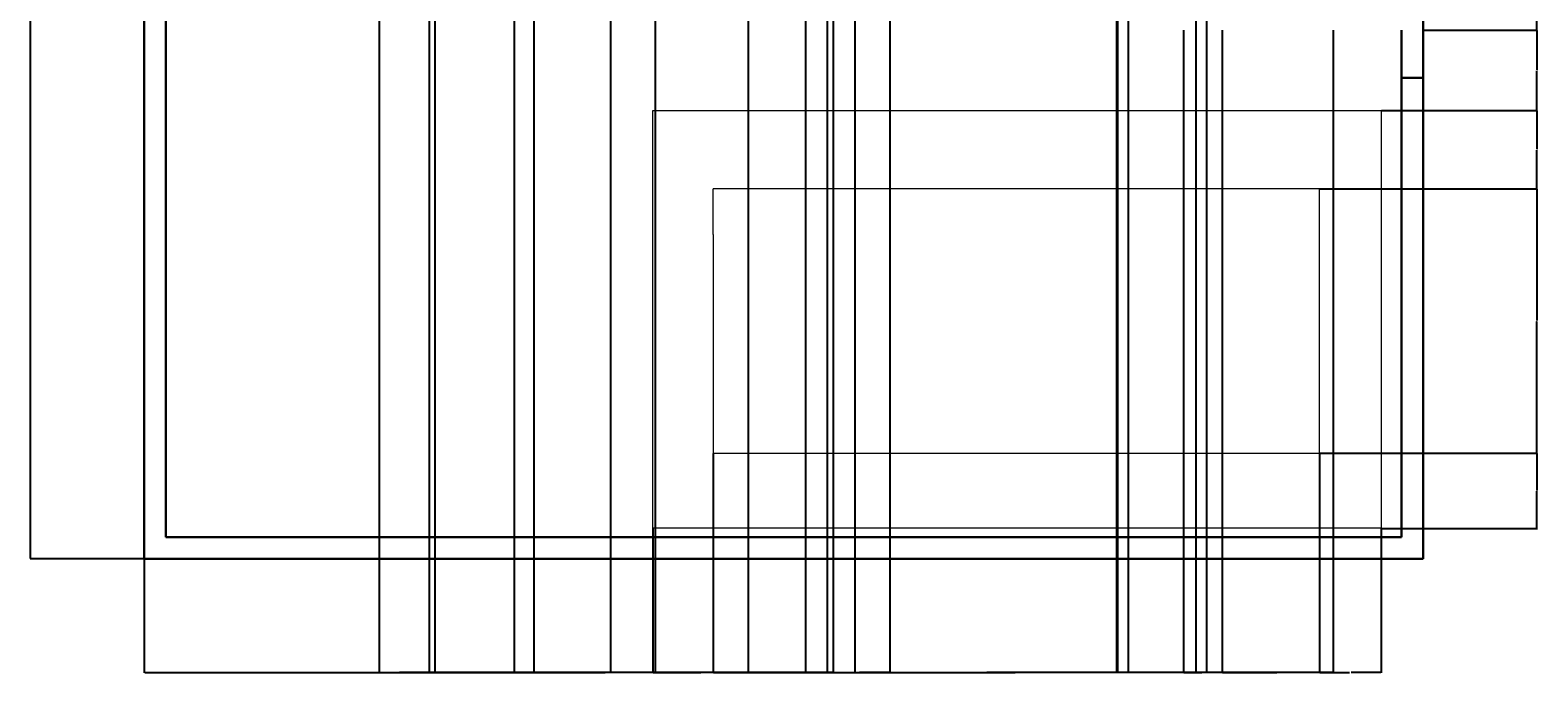
# Model space of a CAD drawing. Units: inches. Extents: x 1210 to 1836, y 84 to 1122.
# Tile 1 of 5: x 1210 to 1836, y 84 to 351. Entities that reach past the tile are written whole.
import ezdxf

# ---------------------------------------------------------------- set-up
doc = ezdxf.new("R2010")
doc.units = ezdxf.units.IN
doc.header["$MEASUREMENT"] = 0
for name, color, linetype, lineweight in [('A-ANNO-DIMS', 2, 'Continuous', 18), ('C-PROP', 32, 'Continuous', 30), ('C-SITE', 32, 'Continuous', 18)]:
    doc.layers.add(name, color=color, linetype=linetype, lineweight=lineweight)
doc.styles.get("Standard").update_dxf_attribs({"font": 'arial.ttf'})
doc.dimstyles.get("Standard").update_dxf_attribs({"dimtxt": 0.18, "dimasz": 0.18, "dimexe": 0.18, "dimexo": 0.0625, "dimgap": 0.09, "dimtad": 0, "dimtih": 1, "dimtoh": 1, "dimdec": 4, "dimzin": 0, "dimdsep": 46, "dimtxsty": 'Standard', "dimcen": 0.09, "dimadec": 0, "dimazin": 0, "dimtfac": 1, "dimtdec": 4, "dimtofl": 0, "dimtmove": 0, "dimatfit": 3, "dimfxl": 1, "dimtolj": 1, "dimtzin": 0, "dimarcsym": 0})

# ---------------------------------------------------------------- blocks, each defined once
blk = doc.blocks.new('*D23')
at = {"layer": 'A-ANNO-DIMS', "color": 0, "lineweight": -2, "transparency": 16777216}
for p, q in [((1257.26, 1074.21), (1209.97, 1074.21)), ((1210.15, 1074.03), (1210.15, 602.9)), ((1210.15, 131.39), (1210.15, 602.53)), ((1257.26, 131.21), (1209.97, 131.21))]:
    blk.add_line(p, q, dxfattribs=at)
at = {"layer": 'A-ANNO-DIMS', "color": 0, "transparency": 16777216}
for points in [[(1210.12, 1074.03), (1210.18, 1074.03), (1210.15, 1074.21)], [(1210.12, 131.39), (1210.18, 131.39), (1210.15, 131.21)]]:
    blk.add_solid(points, dxfattribs=at)
at = {"layer": 'Defpoints', "color": 0, "transparency": 16777216}
for p in [(1210.15, 1074.21), (1257.32, 1074.21), (1257.32, 131.21)]:
    blk.add_point(p, dxfattribs=at)
at = {"layer": 'A-ANNO-DIMS', "color": 0, "transparency": 16777216, "insert": (1210.15, 602.71), "char_height": 0.18, "attachment_point": 5}
blk.add_mtext('\\A1;943', dxfattribs=at)
blk = doc.blocks.new('*D27')
at = {"layer": 'A-ANNO-DIMS', "color": 0, "lineweight": -2, "transparency": 16777216}
for p, q in [((1788.39, 590.21), (1835.68, 590.21)), ((1835.5, 590.03), (1835.5, 470.65)), ((1835.5, 350.89), (1835.5, 470.28)), ((1788.39, 350.71), (1835.68, 350.71))]:
    blk.add_line(p, q, dxfattribs=at)
at = {"layer": 'A-ANNO-DIMS', "color": 0, "transparency": 16777216}
for points in [[(1835.47, 590.03), (1835.53, 590.03), (1835.5, 590.21)], [(1835.47, 350.89), (1835.53, 350.89), (1835.5, 350.71)]]:
    blk.add_solid(points, dxfattribs=at)
at = {"layer": 'Defpoints', "color": 0, "transparency": 16777216}
for p in [(1788.32, 590.21), (1788.32, 350.71), (1835.5, 350.71)]:
    blk.add_point(p, dxfattribs=at)
at = {"layer": 'A-ANNO-DIMS', "color": 0, "transparency": 16777216, "insert": (1835.5, 470.46), "char_height": 0.18, "attachment_point": 5}
blk.add_mtext('\\A1;239.5', dxfattribs=at)
blk = doc.blocks.new('*D28')
at = {"layer": 'A-ANNO-DIMS', "color": 0, "lineweight": -2, "transparency": 16777216}
for p, q in [((1468.42, 143.8), (1468.42, 83.86)), ((1257.32, 131.15), (1257.32, 83.86)), ((1257.5, 84.04), (1362.5, 84.04)), ((1468.24, 84.04), (1363.25, 84.04))]:
    blk.add_line(p, q, dxfattribs=at)
at = {"layer": 'A-ANNO-DIMS', "color": 0, "transparency": 16777216}
for points in [[(1257.5, 84.07), (1257.5, 84.01), (1257.32, 84.04)], [(1468.24, 84.07), (1468.24, 84.01), (1468.42, 84.04)]]:
    blk.add_solid(points, dxfattribs=at)
at = {"layer": 'Defpoints', "color": 0, "transparency": 16777216}
for p in [(1468.42, 143.86), (1257.32, 131.21), (1468.42, 84.04)]:
    blk.add_point(p, dxfattribs=at)
at = {"layer": 'A-ANNO-DIMS', "color": 0, "transparency": 16777216, "insert": (1362.87, 84.04), "char_height": 0.18, "attachment_point": 5}
blk.add_mtext('\\A1;211.1', dxfattribs=at)
blk = doc.blocks.new('*D29')
at = {"layer": 'A-ANNO-DIMS', "color": 0, "lineweight": -2, "transparency": 16777216}
for p, q in [((1493.48, 174.99), (1493.48, 83.86)), ((1468.42, 143.8), (1468.42, 83.86)), ((1468.6, 84.04), (1480.56, 84.04)), ((1493.3, 84.04), (1481.35, 84.04))]:
    blk.add_line(p, q, dxfattribs=at)
at = {"layer": 'A-ANNO-DIMS', "color": 0, "transparency": 16777216}
for points in [[(1468.6, 84.07), (1468.6, 84.01), (1468.42, 84.04)], [(1493.3, 84.07), (1493.3, 84.01), (1493.48, 84.04)]]:
    blk.add_solid(points, dxfattribs=at)
at = {"layer": 'Defpoints', "color": 0, "transparency": 16777216}
for p in [(1493.48, 175.05), (1468.42, 143.86), (1493.48, 84.04)]:
    blk.add_point(p, dxfattribs=at)
at = {"layer": 'A-ANNO-DIMS', "color": 0, "transparency": 16777216, "insert": (1480.95, 84.04), "char_height": 0.18, "attachment_point": 5}
blk.add_mtext('\\A1;25.06', dxfattribs=at)
blk = doc.blocks.new('*D30')
at = {"layer": 'A-ANNO-DIMS', "color": 0, "lineweight": -2, "transparency": 16777216}
for p, q in [((1493.48, 174.99), (1493.48, 83.86)), ((1745.25, 174.99), (1745.25, 83.86)), ((1493.66, 84.04), (1618.9, 84.04)), ((1745.07, 84.04), (1619.83, 84.04))]:
    blk.add_line(p, q, dxfattribs=at)
at = {"layer": 'A-ANNO-DIMS', "color": 0, "transparency": 16777216}
for points in [[(1493.66, 84.07), (1493.66, 84.01), (1493.48, 84.04)], [(1745.07, 84.07), (1745.07, 84.01), (1745.25, 84.04)]]:
    blk.add_solid(points, dxfattribs=at)
at = {"layer": 'Defpoints', "color": 0, "transparency": 16777216}
for p in [(1493.48, 175.05), (1745.25, 175.05), (1745.25, 84.04)]:
    blk.add_point(p, dxfattribs=at)
at = {"layer": 'A-ANNO-DIMS', "color": 0, "transparency": 16777216, "insert": (1619.37, 84.04), "char_height": 0.18, "attachment_point": 5}
blk.add_mtext('\\A1;251.77', dxfattribs=at)
blk = doc.blocks.new('*D31')
at = {"layer": 'A-ANNO-DIMS', "color": 0, "lineweight": -2, "transparency": 16777216}
for p, q in [((1745.25, 174.99), (1745.25, 83.86)), ((1770.85, 143.8), (1770.85, 83.86)), ((1745.43, 84.04), (1757.73, 84.04)), ((1770.67, 84.04), (1758.38, 84.04))]:
    blk.add_line(p, q, dxfattribs=at)
at = {"layer": 'A-ANNO-DIMS', "color": 0, "transparency": 16777216}
for points in [[(1745.43, 84.07), (1745.43, 84.01), (1745.25, 84.04)], [(1770.67, 84.07), (1770.67, 84.01), (1770.85, 84.04)]]:
    blk.add_solid(points, dxfattribs=at)
at = {"layer": 'Defpoints', "color": 0, "transparency": 16777216}
for p in [(1745.25, 175.05), (1770.85, 143.86), (1770.85, 84.04)]:
    blk.add_point(p, dxfattribs=at)
at = {"layer": 'A-ANNO-DIMS', "color": 0, "transparency": 16777216, "insert": (1758.05, 84.04), "char_height": 0.18, "attachment_point": 5}
blk.add_mtext('\\A1;25.6', dxfattribs=at)
blk = doc.blocks.new('*D32')
at = {"layer": 'A-ANNO-DIMS', "color": 0, "lineweight": -2, "transparency": 16777216}
for p, q in [((1745.31, 175.05), (1835.68, 175.05)), ((1835.5, 174.87), (1835.5, 159.64)), ((1835.5, 144.04), (1835.5, 159.28)), ((1770.92, 143.86), (1835.68, 143.86))]:
    blk.add_line(p, q, dxfattribs=at)
at = {"layer": 'A-ANNO-DIMS', "color": 0, "transparency": 16777216}
for points in [[(1835.47, 174.87), (1835.53, 174.87), (1835.5, 175.05)], [(1835.47, 144.04), (1835.53, 144.04), (1835.5, 143.86)]]:
    blk.add_solid(points, dxfattribs=at)
at = {"layer": 'Defpoints', "color": 0, "transparency": 16777216}
for p in [(1745.25, 175.05), (1835.5, 175.05), (1770.85, 143.86)]:
    blk.add_point(p, dxfattribs=at)
at = {"layer": 'A-ANNO-DIMS', "color": 0, "transparency": 16777216, "insert": (1835.5, 159.46), "char_height": 0.18, "attachment_point": 5}
blk.add_mtext('\\A1;31.19', dxfattribs=at)
blk = doc.blocks.new('*D33')
at = {"layer": 'A-ANNO-DIMS', "color": 0, "lineweight": -2, "transparency": 16777216}
for p, q in [((1745.31, 284.89), (1835.68, 284.89)), ((1835.5, 284.71), (1835.5, 230.15)), ((1835.5, 175.23), (1835.5, 229.79)), ((1745.31, 175.05), (1835.68, 175.05))]:
    blk.add_line(p, q, dxfattribs=at)
at = {"layer": 'A-ANNO-DIMS', "color": 0, "transparency": 16777216}
for points in [[(1835.47, 284.71), (1835.53, 284.71), (1835.5, 284.89)], [(1835.47, 175.23), (1835.53, 175.23), (1835.5, 175.05)]]:
    blk.add_solid(points, dxfattribs=at)
at = {"layer": 'Defpoints', "color": 0, "transparency": 16777216}
for p in [(1745.25, 284.89), (1835.5, 284.89), (1745.25, 175.05)]:
    blk.add_point(p, dxfattribs=at)
at = {"layer": 'A-ANNO-DIMS', "color": 0, "transparency": 16777216, "insert": (1835.5, 229.97), "char_height": 0.18, "attachment_point": 5}
blk.add_mtext('\\A1;109.83', dxfattribs=at)
blk = doc.blocks.new('*D34')
at = {"layer": 'A-ANNO-DIMS', "color": 0, "lineweight": -2, "transparency": 16777216}
for p, q in [((1770.92, 317.37), (1835.68, 317.37)), ((1835.5, 317.19), (1835.5, 301.31)), ((1835.5, 285.07), (1835.5, 300.94)), ((1745.31, 284.89), (1835.68, 284.89))]:
    blk.add_line(p, q, dxfattribs=at)
at = {"layer": 'A-ANNO-DIMS', "color": 0, "transparency": 16777216}
for points in [[(1835.47, 317.19), (1835.53, 317.19), (1835.5, 317.37)], [(1835.47, 285.07), (1835.53, 285.07), (1835.5, 284.89)]]:
    blk.add_solid(points, dxfattribs=at)
at = {"layer": 'Defpoints', "color": 0, "transparency": 16777216}
for p in [(1770.85, 317.37), (1835.5, 317.37), (1745.25, 284.89)]:
    blk.add_point(p, dxfattribs=at)
at = {"layer": 'A-ANNO-DIMS', "color": 0, "transparency": 16777216, "insert": (1835.5, 301.13), "char_height": 0.18, "attachment_point": 5}
blk.add_mtext('\\A1;32.48', dxfattribs=at)
blk = doc.blocks.new('*D35')
at = {"layer": 'A-ANNO-DIMS', "color": 0, "lineweight": -2, "transparency": 16777216}
for p, q in [((1788.39, 350.71), (1835.68, 350.71)), ((1835.5, 350.53), (1835.5, 334.22)), ((1835.5, 317.55), (1835.5, 333.86)), ((1770.92, 317.37), (1835.68, 317.37))]:
    blk.add_line(p, q, dxfattribs=at)
at = {"layer": 'A-ANNO-DIMS', "color": 0, "transparency": 16777216}
for points in [[(1835.47, 350.53), (1835.53, 350.53), (1835.5, 350.71)], [(1835.47, 317.55), (1835.53, 317.55), (1835.5, 317.37)]]:
    blk.add_solid(points, dxfattribs=at)
at = {"layer": 'Defpoints', "color": 0, "transparency": 16777216}
for p in [(1788.32, 350.71), (1835.5, 350.71), (1770.85, 317.37)]:
    blk.add_point(p, dxfattribs=at)
at = {"layer": 'A-ANNO-DIMS', "color": 0, "transparency": 16777216, "insert": (1835.5, 334.04), "char_height": 0.18, "attachment_point": 5}
blk.add_mtext('\\A1;33.35', dxfattribs=at)
blk = doc.blocks.new('*D36')
at = {"layer": 'A-ANNO-DIMS', "color": 0, "lineweight": -2, "transparency": 16777216}
for p, q in [((1552.32, 840.82), (1552.32, 83.86)), ((1661.32, 840.82), (1661.32, 83.86)), ((1552.5, 84.04), (1606.54, 84.04)), ((1661.14, 84.04), (1607.1, 84.04))]:
    blk.add_line(p, q, dxfattribs=at)
at = {"layer": 'A-ANNO-DIMS', "color": 0, "transparency": 16777216}
for points in [[(1552.5, 84.07), (1552.5, 84.01), (1552.32, 84.04)], [(1661.14, 84.07), (1661.14, 84.01), (1661.32, 84.04)]]:
    blk.add_solid(points, dxfattribs=at)
at = {"layer": 'Defpoints', "color": 0, "transparency": 16777216}
for p in [(1552.32, 840.89), (1661.32, 840.89), (1661.32, 84.04)]:
    blk.add_point(p, dxfattribs=at)
at = {"layer": 'A-ANNO-DIMS', "color": 0, "transparency": 16777216, "insert": (1606.82, 84.04), "char_height": 0.18, "attachment_point": 5}
blk.add_mtext('\\A1;109', dxfattribs=at)
blk = doc.blocks.new('*D39')
at = {"layer": 'A-ANNO-DIMS', "color": 0, "lineweight": -2, "transparency": 16777216}
for p, q in [((1354.82, 773.15), (1354.82, 83.86)), ((1543.32, 773.15), (1543.32, 83.86)), ((1355, 84.04), (1448.69, 84.04)), ((1543.14, 84.04), (1449.46, 84.04))]:
    blk.add_line(p, q, dxfattribs=at)
at = {"layer": 'A-ANNO-DIMS', "color": 0, "transparency": 16777216}
for points in [[(1355, 84.07), (1355, 84.01), (1354.82, 84.04)], [(1543.14, 84.07), (1543.14, 84.01), (1543.32, 84.04)]]:
    blk.add_solid(points, dxfattribs=at)
at = {"layer": 'Defpoints', "color": 0, "transparency": 16777216}
for p in [(1354.82, 773.21), (1543.32, 773.21), (1543.32, 84.04)]:
    blk.add_point(p, dxfattribs=at)
at = {"layer": 'A-ANNO-DIMS', "color": 0, "transparency": 16777216, "insert": (1449.07, 84.04), "char_height": 0.18, "attachment_point": 5}
blk.add_mtext('\\A1;188.5', dxfattribs=at)
blk = doc.blocks.new('*D47')
at = {"layer": 'A-ANNO-DIMS', "color": 0, "lineweight": -2, "transparency": 16777216}
for p, q in [((1375.61, 773.15), (1375.61, 83.86)), ((1419.01, 773.15), (1419.01, 83.86)), ((1375.79, 84.04), (1396.98, 84.04)), ((1418.83, 84.04), (1397.64, 84.04))]:
    blk.add_line(p, q, dxfattribs=at)
at = {"layer": 'A-ANNO-DIMS', "color": 0, "transparency": 16777216}
for points in [[(1375.79, 84.07), (1375.79, 84.01), (1375.61, 84.04)], [(1418.83, 84.07), (1418.83, 84.01), (1419.01, 84.04)]]:
    blk.add_solid(points, dxfattribs=at)
at = {"layer": 'Defpoints', "color": 0, "transparency": 16777216}
for p in [(1375.61, 773.21), (1419.01, 773.21), (1419.01, 84.04)]:
    blk.add_point(p, dxfattribs=at)
at = {"layer": 'A-ANNO-DIMS', "color": 0, "transparency": 16777216, "insert": (1397.31, 84.04), "char_height": 0.18, "attachment_point": 5}
blk.add_mtext('\\A1;43.4', dxfattribs=at)
blk = doc.blocks.new('*D48')
at = {"layer": 'A-ANNO-DIMS', "color": 0, "lineweight": -2, "transparency": 16777216}
for p, q in [((1419.01, 773.15), (1419.01, 83.86)), ((1450.89, 772.94), (1450.89, 83.86)), ((1419.19, 84.04), (1434.55, 84.04)), ((1450.71, 84.04), (1435.34, 84.04))]:
    blk.add_line(p, q, dxfattribs=at)
at = {"layer": 'A-ANNO-DIMS', "color": 0, "transparency": 16777216}
for points in [[(1419.19, 84.07), (1419.19, 84.01), (1419.01, 84.04)], [(1450.71, 84.07), (1450.71, 84.01), (1450.89, 84.04)]]:
    blk.add_solid(points, dxfattribs=at)
at = {"layer": 'Defpoints', "color": 0, "transparency": 16777216}
for p in [(1419.01, 773.21), (1450.89, 773), (1450.89, 84.04)]:
    blk.add_point(p, dxfattribs=at)
at = {"layer": 'A-ANNO-DIMS', "color": 0, "transparency": 16777216, "insert": (1434.95, 84.04), "char_height": 0.18, "attachment_point": 5}
blk.add_mtext('\\A1;31.88', dxfattribs=at)
blk = doc.blocks.new('*D57')
at = {"layer": 'A-ANNO-DIMS', "color": 0, "lineweight": -2, "transparency": 16777216}
for p, q in [((1552.32, 764.15), (1552.32, 83.86)), ((1665.82, 764.15), (1665.82, 83.86)), ((1552.5, 84.04), (1608.69, 84.04)), ((1665.64, 84.04), (1609.46, 84.04))]:
    blk.add_line(p, q, dxfattribs=at)
at = {"layer": 'A-ANNO-DIMS', "color": 0, "transparency": 16777216}
for points in [[(1552.5, 84.07), (1552.5, 84.01), (1552.32, 84.04)], [(1665.64, 84.07), (1665.64, 84.01), (1665.82, 84.04)]]:
    blk.add_solid(points, dxfattribs=at)
at = {"layer": 'Defpoints', "color": 0, "transparency": 16777216}
for p in [(1552.32, 764.21), (1665.82, 764.21), (1665.82, 84.04)]:
    blk.add_point(p, dxfattribs=at)
at = {"layer": 'A-ANNO-DIMS', "color": 0, "transparency": 16777216, "insert": (1609.07, 84.04), "char_height": 0.18, "attachment_point": 5}
blk.add_mtext('\\A1;113.5', dxfattribs=at)
blk = doc.blocks.new('*D66')
at = {"layer": 'A-ANNO-DIMS', "color": 0, "lineweight": -2, "transparency": 16777216}
for p, q in [((1508.09, 392.15), (1508.09, 83.86)), ((1531.82, 392.15), (1531.82, 83.86)), ((1508.27, 84.04), (1519.56, 84.04)), ((1531.64, 84.04), (1520.35, 84.04))]:
    blk.add_line(p, q, dxfattribs=at)
at = {"layer": 'A-ANNO-DIMS', "color": 0, "transparency": 16777216}
for points in [[(1508.27, 84.07), (1508.27, 84.01), (1508.09, 84.04)], [(1531.64, 84.07), (1531.64, 84.01), (1531.82, 84.04)]]:
    blk.add_solid(points, dxfattribs=at)
at = {"layer": 'Defpoints', "color": 0, "transparency": 16777216}
for p in [(1508.09, 392.21), (1531.82, 392.21), (1531.82, 84.04)]:
    blk.add_point(p, dxfattribs=at)
at = {"layer": 'A-ANNO-DIMS', "color": 0, "transparency": 16777216, "insert": (1519.96, 84.04), "char_height": 0.18, "attachment_point": 5}
blk.add_mtext('\\A1;23.73', dxfattribs=at)
blk = doc.blocks.new('*D67')
at = {"layer": 'A-ANNO-DIMS', "color": 0, "lineweight": -2, "transparency": 16777216}
for p, q in [((1469.4, 392.15), (1469.4, 83.86)), ((1508.09, 392.15), (1508.09, 83.86)), ((1469.58, 84.04), (1488.42, 84.04)), ((1507.91, 84.04), (1489.07, 84.04))]:
    blk.add_line(p, q, dxfattribs=at)
at = {"layer": 'A-ANNO-DIMS', "color": 0, "transparency": 16777216}
for points in [[(1469.58, 84.07), (1469.58, 84.01), (1469.4, 84.04)], [(1507.91, 84.07), (1507.91, 84.01), (1508.09, 84.04)]]:
    blk.add_solid(points, dxfattribs=at)
at = {"layer": 'Defpoints', "color": 0, "transparency": 16777216}
for p in [(1469.4, 392.21), (1508.09, 392.21), (1508.09, 84.04)]:
    blk.add_point(p, dxfattribs=at)
at = {"layer": 'A-ANNO-DIMS', "color": 0, "transparency": 16777216, "insert": (1488.75, 84.04), "char_height": 0.18, "attachment_point": 5}
blk.add_mtext('\\A1;38.7', dxfattribs=at)
blk = doc.blocks.new('*D68')
at = {"layer": 'A-ANNO-DIMS', "color": 0, "lineweight": -2, "transparency": 16777216}
for p, q in [((1540.82, 392.15), (1540.82, 83.86)), ((1566.82, 392.15), (1566.82, 83.86)), ((1541, 84.04), (1553.42, 84.04)), ((1566.64, 84.04), (1554.22, 84.04))]:
    blk.add_line(p, q, dxfattribs=at)
at = {"layer": 'A-ANNO-DIMS', "color": 0, "transparency": 16777216}
for points in [[(1541, 84.07), (1541, 84.01), (1540.82, 84.04)], [(1566.64, 84.07), (1566.64, 84.01), (1566.82, 84.04)]]:
    blk.add_solid(points, dxfattribs=at)
at = {"layer": 'Defpoints', "color": 0, "transparency": 16777216}
for p in [(1540.82, 392.21), (1566.82, 392.21), (1566.82, 84.04)]:
    blk.add_point(p, dxfattribs=at)
at = {"layer": 'A-ANNO-DIMS', "color": 0, "transparency": 16777216, "insert": (1553.82, 84.04), "char_height": 0.18, "attachment_point": 5}
blk.add_mtext('\\A1;25.99', dxfattribs=at)
blk = doc.blocks.new('*D69')
at = {"layer": 'A-ANNO-DIMS', "color": 0, "lineweight": -2, "transparency": 16777216}
for p, q in [((1566.82, 392.15), (1566.82, 83.86)), ((1660.99, 392.15), (1660.99, 83.86)), ((1567, 84.04), (1613.51, 84.04)), ((1660.81, 84.04), (1614.29, 84.04))]:
    blk.add_line(p, q, dxfattribs=at)
at = {"layer": 'A-ANNO-DIMS', "color": 0, "transparency": 16777216}
for points in [[(1567, 84.07), (1567, 84.01), (1566.82, 84.04)], [(1660.81, 84.07), (1660.81, 84.01), (1660.99, 84.04)]]:
    blk.add_solid(points, dxfattribs=at)
at = {"layer": 'Defpoints', "color": 0, "transparency": 16777216}
for p in [(1566.82, 392.21), (1660.99, 392.21), (1660.99, 84.04)]:
    blk.add_point(p, dxfattribs=at)
at = {"layer": 'A-ANNO-DIMS', "color": 0, "transparency": 16777216, "insert": (1613.9, 84.04), "char_height": 0.18, "attachment_point": 5}
blk.add_mtext('\\A1;94.17', dxfattribs=at)
blk = doc.blocks.new('*D70')
at = {"layer": 'A-ANNO-DIMS', "color": 0, "lineweight": -2, "transparency": 16777216}
for p, q in [((1688.72, 350.65), (1688.72, 83.86)), ((1704.83, 350.65), (1704.83, 83.86)), ((1688.9, 84.04), (1696.32, 84.04)), ((1704.65, 84.04), (1697.23, 84.04))]:
    blk.add_line(p, q, dxfattribs=at)
at = {"layer": 'A-ANNO-DIMS', "color": 0, "transparency": 16777216}
for points in [[(1688.9, 84.07), (1688.9, 84.01), (1688.72, 84.04)], [(1704.65, 84.07), (1704.65, 84.01), (1704.83, 84.04)]]:
    blk.add_solid(points, dxfattribs=at)
at = {"layer": 'Defpoints', "color": 0, "transparency": 16777216}
for p in [(1688.72, 350.71), (1704.83, 350.71), (1704.83, 84.04)]:
    blk.add_point(p, dxfattribs=at)
at = {"layer": 'A-ANNO-DIMS', "color": 0, "transparency": 16777216, "insert": (1696.78, 84.04), "char_height": 0.18, "attachment_point": 5}
blk.add_mtext('\\A1;16.107', dxfattribs=at)
blk = doc.blocks.new('*D71')
at = {"layer": 'A-ANNO-DIMS', "color": 0, "lineweight": -2, "transparency": 16777216}
for p, q in [((1704.83, 350.65), (1704.83, 83.86)), ((1750.9, 350.65), (1750.9, 83.86)), ((1705.01, 84.04), (1727.47, 84.04)), ((1750.72, 84.04), (1728.26, 84.04))]:
    blk.add_line(p, q, dxfattribs=at)
at = {"layer": 'A-ANNO-DIMS', "color": 0, "transparency": 16777216}
for points in [[(1705.01, 84.07), (1705.01, 84.01), (1704.83, 84.04)], [(1750.72, 84.07), (1750.72, 84.01), (1750.9, 84.04)]]:
    blk.add_solid(points, dxfattribs=at)
at = {"layer": 'Defpoints', "color": 0, "transparency": 16777216}
for p in [(1704.83, 350.71), (1750.9, 350.71), (1750.9, 84.04)]:
    blk.add_point(p, dxfattribs=at)
at = {"layer": 'A-ANNO-DIMS', "color": 0, "transparency": 16777216, "insert": (1727.86, 84.04), "char_height": 0.18, "attachment_point": 5}
blk.add_mtext('\\A1;46.07', dxfattribs=at)
blk = doc.blocks.new('*D74')
at = {"layer": 'A-ANNO-DIMS', "color": 0, "lineweight": -2, "transparency": 16777216}
for p, q in [((1377.99, 581.15), (1377.99, 83.86)), ((1410.82, 581.15), (1410.82, 83.86)), ((1378.17, 84.04), (1394.01, 84.04)), ((1410.64, 84.04), (1394.8, 84.04))]:
    blk.add_line(p, q, dxfattribs=at)
at = {"layer": 'A-ANNO-DIMS', "color": 0, "transparency": 16777216}
for points in [[(1378.17, 84.07), (1378.17, 84.01), (1377.99, 84.04)], [(1410.64, 84.07), (1410.64, 84.01), (1410.82, 84.04)]]:
    blk.add_solid(points, dxfattribs=at)
at = {"layer": 'Defpoints', "color": 0, "transparency": 16777216}
for p in [(1377.99, 581.21), (1410.82, 581.21), (1410.82, 84.04)]:
    blk.add_point(p, dxfattribs=at)
at = {"layer": 'A-ANNO-DIMS', "color": 0, "transparency": 16777216, "insert": (1394.4, 84.04), "char_height": 0.18, "attachment_point": 5}
blk.add_mtext('\\A1;32.84', dxfattribs=at)
blk = doc.blocks.new('*D75')
at = {"layer": 'A-ANNO-DIMS', "color": 0, "lineweight": -2, "transparency": 16777216}
for p, q in [((1410.82, 575.15), (1410.82, 83.86)), ((1450.82, 575.15), (1450.82, 83.86)), ((1411, 84.04), (1430.6, 84.04)), ((1450.64, 84.04), (1431.05, 84.04))]:
    blk.add_line(p, q, dxfattribs=at)
at = {"layer": 'A-ANNO-DIMS', "color": 0, "transparency": 16777216}
for points in [[(1411, 84.07), (1411, 84.01), (1410.82, 84.04)], [(1450.64, 84.07), (1450.64, 84.01), (1450.82, 84.04)]]:
    blk.add_solid(points, dxfattribs=at)
at = {"layer": 'Defpoints', "color": 0, "transparency": 16777216}
for p in [(1410.82, 575.21), (1450.82, 575.21), (1450.82, 84.04)]:
    blk.add_point(p, dxfattribs=at)
at = {"layer": 'A-ANNO-DIMS', "color": 0, "transparency": 16777216, "insert": (1430.82, 84.04), "char_height": 0.18, "attachment_point": 5}
blk.add_mtext('\\A1;40', dxfattribs=at)
blk = doc.blocks.new('*D78')
at = {"layer": 'A-ANNO-DIMS', "color": 0, "lineweight": -2, "transparency": 16777216}
for p, q in [((1693.82, 581.15), (1693.82, 83.86)), ((1698.32, 581.15), (1698.32, 83.86)), ((1694, 84.04), (1695.82, 84.04)), ((1698.14, 84.04), (1696.33, 84.04))]:
    blk.add_line(p, q, dxfattribs=at)
at = {"layer": 'A-ANNO-DIMS', "color": 0, "transparency": 16777216}
for points in [[(1694, 84.07), (1694, 84.01), (1693.82, 84.04)], [(1698.14, 84.07), (1698.14, 84.01), (1698.32, 84.04)]]:
    blk.add_solid(points, dxfattribs=at)
at = {"layer": 'Defpoints', "color": 0, "transparency": 16777216}
for p in [(1693.82, 581.21), (1698.32, 581.21), (1698.32, 84.04)]:
    blk.add_point(p, dxfattribs=at)
at = {"layer": 'A-ANNO-DIMS', "color": 0, "transparency": 16777216, "insert": (1696.07, 84.04), "char_height": 0.18, "attachment_point": 5}
blk.add_mtext('\\A1;4.5', dxfattribs=at)

msp = doc.modelspace()

# ---------------------------------------------------------------- linework, layer by layer
at = {"layer": 'C-PROP'}
for p, q in [((1257.3239, 131.214), (1257.3239, 1074.214)), ((1788.3239, 1074.214), (1788.3239, 131.214)), ((1266.3239, 140.214), (1266.3239, 764.214)), ((1779.3239, 350.714), (1779.3239, 140.214)), ((1779.3239, 330.9444), (1788.3239, 330.9444)), ((1779.3239, 299.7489), (1779.3239, 261.988)), ((1779.3239, 140.214), (1266.3239, 140.214)), ((1450.8239, 140.214), (1468.424, 140.214)), ((1788.3239, 131.214), (1257.3239, 131.214))]:
    msp.add_line(p, q, dxfattribs=at)
at = {"layer": 'C-SITE'}
for p, q in [((1468.424, 143.8648), (1468.424, 317.366)), ((1468.424, 317.366), (1770.853, 317.366)), ((1770.853, 317.366), (1770.853, 143.8648)), ((1745.2514, 284.8863), (1493.4841, 284.8863)), ((1493.4841, 265.8707), (1493.4841, 284.8863)), ((1745.2514, 175.0525), (1745.2514, 284.8863)), ((1493.4841, 265.8707), (1493.4841, 175.0525)), ((1493.4841, 175.0525), (1745.2514, 175.0525)), ((1770.853, 143.8648), (1468.424, 143.8648))]:
    msp.add_line(p, q, dxfattribs=at)

# ---------------------------------------------------------------- dimensions: what is measured, and where the dimension line sits
at = {"layer": 'A-ANNO-DIMS'}
for base, p1, p2, override, picture, middle in [((1210.1489, 1074.214), (1257.3239, 131.214), (1257.3239, 1074.214), {"dimdec": 0, "dimlfac": 1, "dimrnd": 0, "dimzin": 0, "dimdsep": 46, "dimlunit": 2}, '*D23', (1210.1489, 602.714)), ((1835.4989, 350.714), (1788.3239, 590.214), (1788.3239, 350.714), {"dimdec": 1, "dimlfac": 1, "dimrnd": 0, "dimzin": 0, "dimdsep": 46, "dimlunit": 2}, '*D27', (1835.4989, 470.464)), ((1835.4989, 350.714), (1770.853, 317.366), (1788.3239, 350.714), {"dimdec": 2, "dimlfac": 1, "dimrnd": 0, "dimzin": 0, "dimdsep": 46, "dimlunit": 2}, '*D35', (1835.4989, 334.04)), ((1835.4989, 317.366), (1745.2514, 284.8863), (1770.853, 317.366), {"dimdec": 2, "dimlfac": 1, "dimrnd": 0, "dimzin": 0, "dimdsep": 46, "dimlunit": 2}, '*D34', (1835.4989, 301.1261)), ((1835.4989, 284.8863), (1745.2514, 175.0525), (1745.2514, 284.8863), {"dimdec": 2, "dimlfac": 1, "dimrnd": 0, "dimzin": 0, "dimdsep": 46, "dimlunit": 2}, '*D33', (1835.4989, 229.9694)), ((1835.4989, 175.0525), (1770.853, 143.8648), (1745.2514, 175.0525), {"dimdec": 2, "dimlfac": 1, "dimrnd": 0, "dimzin": 0, "dimdsep": 46, "dimlunit": 2}, '*D32', (1835.4989, 159.4587))]:
    dim = msp.add_linear_dim(base=base, p1=p1, p2=p2, angle=90, dimstyle='Standard', override=override, dxfattribs=at)
    dim.commit()
    dim.dimension.update_dxf_attribs({"geometry": picture, "text_midpoint": middle})
for base, p1, p2, override, picture, middle in [((1661.3239, 84.039), (1552.3239, 840.8861), (1661.3239, 840.8861), {"dimdec": 0, "dimlfac": 1, "dimrnd": 0, "dimzin": 0, "dimdsep": 46, "dimlunit": 2}, '*D36', (1606.8239, 84.039)), ((1543.3239, 84.039), (1354.8239, 773.214), (1543.3239, 773.214), {"dimdec": 1, "dimlfac": 1, "dimrnd": 0, "dimzin": 0, "dimdsep": 46, "dimlunit": 2}, '*D39', (1449.0739, 84.039)), ((1419.0081, 84.039), (1375.6096, 773.214), (1419.0081, 773.214), {"dimdec": 1, "dimlfac": 1, "dimrnd": 0, "dimzin": 0, "dimdsep": 46, "dimlunit": 2}, '*D47', (1397.3088, 84.039)), ((1450.8864, 84.039), (1419.0081, 773.214), (1450.8864, 773.0031), {"dimdec": 2, "dimlfac": 1, "dimrnd": 0, "dimzin": 0, "dimdsep": 46, "dimlunit": 2}, '*D48', (1434.9472, 84.039)), ((1665.8239, 84.039), (1552.3239, 764.214), (1665.8239, 764.214), {"dimdec": 1, "dimlfac": 1, "dimrnd": 0, "dimzin": 0, "dimdsep": 46, "dimlunit": 2}, '*D57', (1609.0739, 84.039)), ((1410.8239, 84.039), (1377.9853, 581.214), (1410.8239, 581.214), {"dimdec": 2, "dimlfac": 1, "dimrnd": 0, "dimzin": 0, "dimdsep": 46, "dimlunit": 2}, '*D74', (1394.4046, 84.039)), ((1698.3239, 84.039), (1693.8239, 581.214), (1698.3239, 581.214), {"dimdec": 1, "dimlfac": 1, "dimrnd": 0, "dimzin": 0, "dimdsep": 46, "dimlunit": 2}, '*D78', (1696.0739, 84.039)), ((1450.8239, 84.039), (1410.8239, 575.214), (1450.8239, 575.214), {"dimdec": 0, "dimlfac": 1, "dimrnd": 0, "dimzin": 0, "dimdsep": 46, "dimlunit": 2}, '*D75', (1430.8239, 84.039)), ((1508.0938, 84.039), (1469.397, 392.214), (1508.0938, 392.214), {"dimdec": 1, "dimlfac": 1, "dimrnd": 0, "dimzin": 0, "dimdsep": 46, "dimlunit": 2}, '*D67', (1488.7454, 84.039)), ((1531.8239, 84.039), (1508.0938, 392.214), (1531.8239, 392.214), {"dimdec": 2, "dimlfac": 1, "dimrnd": 0, "dimzin": 0, "dimdsep": 46, "dimlunit": 2}, '*D66', (1519.9588, 84.039)), ((1566.8155, 84.039), (1540.8239, 392.214), (1566.8155, 392.214), {"dimdec": 2, "dimlfac": 1, "dimrnd": 0, "dimzin": 0, "dimdsep": 46, "dimlunit": 2}, '*D68', (1553.8197, 84.039)), ((1660.9867, 84.039), (1566.8155, 392.214), (1660.9867, 392.214), {"dimdec": 2, "dimlfac": 1, "dimrnd": 0, "dimzin": 0, "dimdsep": 46, "dimlunit": 2}, '*D69', (1613.9011, 84.039)), ((1704.8288, 84.039), (1688.7218, 350.714), (1704.8288, 350.714), {"dimdec": 3, "dimlfac": 1, "dimrnd": 0, "dimzin": 0, "dimdsep": 46, "dimlunit": 2}, '*D70', (1696.7753, 84.039)), ((1750.8976, 84.039), (1704.8288, 350.714), (1750.8976, 350.714), {"dimdec": 2, "dimlfac": 1, "dimrnd": 0, "dimzin": 0, "dimdsep": 46, "dimlunit": 2}, '*D71', (1727.8632, 84.039)), ((1493.4841, 84.039), (1468.424, 143.8648), (1493.4841, 175.0525), {"dimdec": 2, "dimlfac": 1, "dimrnd": 0, "dimzin": 0, "dimdsep": 46, "dimlunit": 2}, '*D29', (1480.9541, 84.039)), ((1745.2514, 84.039), (1493.4841, 175.0525), (1745.2514, 175.0525), {"dimdec": 2, "dimlfac": 1, "dimrnd": 0, "dimzin": 0, "dimdsep": 46, "dimlunit": 2}, '*D30', (1619.3677, 84.039)), ((1770.853, 84.039), (1745.2514, 175.0525), (1770.853, 143.8648), {"dimdec": 1, "dimlfac": 1, "dimrnd": 0, "dimzin": 0, "dimdsep": 46, "dimlunit": 2}, '*D31', (1758.0522, 84.039)), ((1468.424, 84.039), (1257.3239, 131.214), (1468.424, 143.8648), {"dimdec": 1, "dimlfac": 1, "dimrnd": 0, "dimzin": 0, "dimdsep": 46, "dimlunit": 2}, '*D28', (1362.874, 84.039))]:
    dim = msp.add_linear_dim(base=base, p1=p1, p2=p2, dimstyle='Standard', override=override, dxfattribs=at)
    dim.commit()
    dim.dimension.update_dxf_attribs({"geometry": picture, "text_midpoint": middle})

doc.saveas('drawing.dxf')
